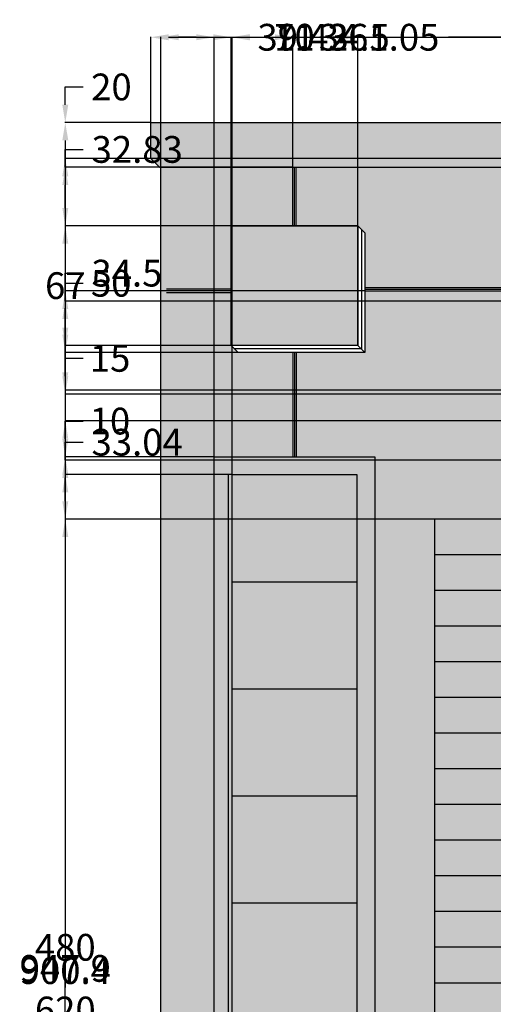
# Model space of a CAD drawing. Units: millimetres. Extents: x 131 to 845, y -20 to 1043.
# Tile 9 of 11: x 137 to 403, y 492 to 1043. Entities that reach past the tile are written whole.
import ezdxf

# ---------------------------------------------------------------- set-up
doc = ezdxf.new("R2010")
doc.units = ezdxf.units.MM
doc.header["$MEASUREMENT"] = 0
for name, color, linetype, lineweight in [('A-ANNO-DIMS', 2, 'Continuous', 18), ('A-ELEV', 7, 'Continuous', 25), ('A-ELEV-PATT', 7, 'Continuous', 13), ('A-GLAZ', 4, 'Continuous', 25), ('A-WALL-PATT', 131, 'Continuous', 13)]:
    doc.layers.add(name, color=color, linetype=linetype, lineweight=lineweight)
doc.styles.get("Standard").update_dxf_attribs({"font": 'arial.ttf'})
doc.dimstyles.get("Standard").update_dxf_attribs({"dimtxt": 15, "dimasz": 10, "dimexe": 0.18, "dimexo": 0.0625, "dimgap": 5, "dimtad": 0, "dimtih": 1, "dimtoh": 1, "dimdec": 0, "dimzin": 0, "dimdsep": 46, "dimtxsty": 'Standard', "dimcen": 5, "dimadec": 0, "dimazin": 0, "dimtfac": 1, "dimtdec": 0, "dimtofl": 0, "dimtmove": 0, "dimatfit": 3, "dimfxl": 1, "dimtolj": 1, "dimtzin": 0, "dimarcsym": 0})

# ---------------------------------------------------------------- blocks, each defined once
blk = doc.blocks.new('*U3')
blk.add_line((0, -70), (0, 0))
blk = doc.blocks.new('*U4')
at = {"layer": 'A-GLAZ', "color": 0, "linetype": 'ByBlock', "lineweight": -2, "transparency": 16777216, "rotation": 270}
for p in [(326.16, 788.43), (326.16, 728.43), (326.16, 668.43), (326.16, 608.43), (326.16, 548.43)]:
    blk.add_blockref('*U3', p, dxfattribs=at)
blk = doc.blocks.new('*U5')
blk.add_line((0, 90), (0, 0))
blk = doc.blocks.new('*U6')
at = {"layer": 'A-ELEV', "color": 0, "linetype": 'ByBlock', "lineweight": -2, "transparency": 16777216, "rotation": 270}
for p in [(369.56, 763.56), (369.56, 743.56), (369.56, 723.56), (369.56, 703.56), (369.56, 683.56), (369.56, 663.56), (369.56, 643.56), (369.56, 623.56), (369.56, 603.56), (369.56, 583.56), (369.56, 563.56), (369.56, 543.56), (369.56, 523.56), (369.56, 503.56), (369.56, 483.56), (369.56, 463.56), (369.56, 443.56), (369.56, 423.56), (369.56, 403.56), (369.56, 383.56), (369.56, 363.56), (369.56, 343.56), (369.56, 323.56), (369.56, 303.56), (369.56, 283.56)]:
    blk.add_blockref('*U5', p, dxfattribs=at)
blk = doc.blocks.new('*D11')
at = {"layer": 'A-ANNO-DIMS', "color": 0, "lineweight": -2, "transparency": 16777216}
for p, q in [((554.73, 464.78), (544.73, 464.78)), ((554.75, 454.78), (554.73, 464.78)), ((550.09, 454.77), (554.93, 454.78)), ((554.78, 433.28), (554.76, 444.78)), ((550.13, 423.27), (554.97, 423.28))]:
    blk.add_line(p, q, dxfattribs=at)
at = {"layer": 'A-ANNO-DIMS', "color": 0, "transparency": 16777216}
for points in [[(556.43, 444.78), (553.1, 444.77), (554.75, 454.78)], [(556.45, 433.28), (553.11, 433.27), (554.79, 423.28)]]:
    blk.add_solid(points, dxfattribs=at)
at = {"layer": 'Defpoints', "color": 0, "transparency": 16777216}
for p in [(550.02, 454.77), (554.75, 454.78), (550.07, 423.27)]:
    blk.add_point(p, dxfattribs=at)
at = {"layer": 'A-ANNO-DIMS', "color": 0, "transparency": 16777216, "insert": (399.96, 464.78), "char_height": 15, "attachment_point": 5}
blk.add_mtext('\\A1;DOOR GLASS PANE 32 TYP.', dxfattribs=at)
blk = doc.blocks.new('*D13')
at = {"layer": 'A-ANNO-DIMS', "color": 0, "lineweight": -2, "transparency": 16777216}
for p, q in [((210.58, 985.73), (210.58, 1033.7)), ((220.58, 1033.52), (444.01, 1033.52)), ((710.53, 1033.52), (487.1, 1033.52)), ((720.53, 818.66), (720.53, 1033.7))]:
    blk.add_line(p, q, dxfattribs=at)
at = {"layer": 'A-ANNO-DIMS', "color": 0, "transparency": 16777216}
for points in [[(220.58, 1035.18), (220.58, 1031.85), (210.58, 1033.52)], [(710.53, 1035.18), (710.53, 1031.85), (720.53, 1033.52)]]:
    blk.add_solid(points, dxfattribs=at)
at = {"layer": 'Defpoints', "color": 0, "transparency": 16777216}
for p in [(720.53, 1033.52), (210.58, 985.67), (720.53, 818.6)]:
    blk.add_point(p, dxfattribs=at)
at = {"layer": 'A-ANNO-DIMS', "color": 0, "transparency": 16777216, "insert": (465.56, 1033.52), "char_height": 15, "attachment_point": 5}
blk.add_mtext('\\A1;510', dxfattribs=at)
blk = doc.blocks.new('*D14')
at = {"layer": 'A-ANNO-DIMS', "color": 0, "lineweight": -2, "transparency": 16777216}
for p, q in [((210.52, 985.67), (162.55, 985.67)), ((162.73, 975.67), (162.73, 524.4)), ((162.73, 47.81), (162.73, 499.08)), ((459.5, 37.81), (162.55, 37.81))]:
    blk.add_line(p, q, dxfattribs=at)
at = {"layer": 'A-ANNO-DIMS', "color": 0, "transparency": 16777216}
for points in [[(161.06, 975.67), (164.4, 975.67), (162.73, 985.67)], [(161.06, 47.81), (164.4, 47.81), (162.73, 37.81)]]:
    blk.add_solid(points, dxfattribs=at)
at = {"layer": 'Defpoints', "color": 0, "transparency": 16777216}
for p in [(162.73, 985.67), (210.58, 985.67), (459.56, 37.81)]:
    blk.add_point(p, dxfattribs=at)
at = {"layer": 'A-ANNO-DIMS', "color": 0, "transparency": 16777216, "insert": (162.73, 511.74), "char_height": 15, "attachment_point": 5}
blk.add_mtext('\\A1;947.9', dxfattribs=at)
blk = doc.blocks.new('*D15')
at = {"layer": 'A-ANNO-DIMS', "color": 0, "lineweight": -2, "transparency": 16777216}
for p, q in [((210.58, 985.73), (210.58, 1033.7)), ((220.58, 1033.52), (304.79, 1033.52)), ((461.63, 1033.52), (377.43, 1033.52)), ((471.63, 965.73), (471.63, 1033.7))]:
    blk.add_line(p, q, dxfattribs=at)
at = {"layer": 'A-ANNO-DIMS', "color": 0, "transparency": 16777216}
for points in [[(220.58, 1035.18), (220.58, 1031.85), (210.58, 1033.52)], [(461.63, 1035.18), (461.63, 1031.85), (471.63, 1033.52)]]:
    blk.add_solid(points, dxfattribs=at)
at = {"layer": 'Defpoints', "color": 0, "transparency": 16777216}
for p in [(471.63, 1033.52), (210.58, 985.67), (471.63, 965.67)]:
    blk.add_point(p, dxfattribs=at)
at = {"layer": 'A-ANNO-DIMS', "color": 0, "transparency": 16777216, "insert": (341.11, 1033.52), "char_height": 15, "attachment_point": 5}
blk.add_mtext('\\A1;261.05', dxfattribs=at)
blk = doc.blocks.new('*D16')
at = {"layer": 'A-ANNO-DIMS', "color": 0, "lineweight": -2, "transparency": 16777216}
for p, q in [((162.73, 995.67), (162.73, 1005.67)), ((162.73, 1005.67), (172.73, 1005.67)), ((210.52, 985.67), (162.55, 985.67)), ((210.52, 965.67), (162.55, 965.67)), ((162.73, 955.67), (162.73, 945.67))]:
    blk.add_line(p, q, dxfattribs=at)
at = {"layer": 'A-ANNO-DIMS', "color": 0, "transparency": 16777216}
for points in [[(161.06, 995.67), (164.4, 995.67), (162.73, 985.67)], [(161.06, 955.67), (164.4, 955.67), (162.73, 965.67)]]:
    blk.add_solid(points, dxfattribs=at)
at = {"layer": 'Defpoints', "color": 0, "transparency": 16777216}
for p in [(162.73, 985.67), (210.58, 985.67), (210.58, 965.67)]:
    blk.add_point(p, dxfattribs=at)
at = {"layer": 'A-ANNO-DIMS', "color": 0, "transparency": 16777216, "insert": (188.58, 1005.67), "char_height": 15, "attachment_point": 5}
blk.add_mtext('\\A1;20', dxfattribs=at)
blk = doc.blocks.new('*D17')
at = {"layer": 'A-ANNO-DIMS', "color": 0, "lineweight": -2, "transparency": 16777216}
for p, q in [((216.17, 960.67), (162.55, 960.67)), ((162.73, 950.67), (162.73, 523.15)), ((162.73, 70.31), (162.73, 497.83)), ((216.17, 60.31), (162.55, 60.31))]:
    blk.add_line(p, q, dxfattribs=at)
at = {"layer": 'A-ANNO-DIMS', "color": 0, "transparency": 16777216}
for points in [[(161.06, 950.67), (164.4, 950.67), (162.73, 960.67)], [(161.06, 70.31), (164.4, 70.31), (162.73, 60.31)]]:
    blk.add_solid(points, dxfattribs=at)
at = {"layer": 'Defpoints', "color": 0, "transparency": 16777216}
for p in [(162.73, 960.67), (216.23, 960.67), (216.23, 60.31)]:
    blk.add_point(p, dxfattribs=at)
at = {"layer": 'A-ANNO-DIMS', "color": 0, "transparency": 16777216, "insert": (162.73, 510.49), "char_height": 15, "attachment_point": 5}
blk.add_mtext('\\A1;900.4', dxfattribs=at)
blk = doc.blocks.new('*D19')
at = {"layer": 'A-ANNO-DIMS', "color": 0, "lineweight": -2, "transparency": 16777216}
for p, q in [((216.23, 960.73), (216.23, 1033.7)), ((226.23, 1033.52), (245.66, 1033.52)), ((255.66, 927.9), (255.66, 1033.7)), ((255.66, 1033.52), (265.66, 1033.52))]:
    blk.add_line(p, q, dxfattribs=at)
at = {"layer": 'A-ANNO-DIMS', "color": 0, "transparency": 16777216}
for points in [[(226.23, 1035.18), (226.23, 1031.85), (216.23, 1033.52)], [(245.66, 1035.18), (245.66, 1031.85), (255.66, 1033.52)]]:
    blk.add_solid(points, dxfattribs=at)
at = {"layer": 'Defpoints', "color": 0, "transparency": 16777216}
for p in [(255.66, 1033.52), (216.23, 960.67), (255.66, 927.83)]:
    blk.add_point(p, dxfattribs=at)
at = {"layer": 'A-ANNO-DIMS', "color": 0, "transparency": 16777216, "insert": (295.96, 1033.52), "char_height": 15, "attachment_point": 5}
blk.add_mtext('\\A1;39.43', dxfattribs=at)
blk = doc.blocks.new('*D20')
at = {"layer": 'A-ANNO-DIMS', "color": 0, "lineweight": -2, "transparency": 16777216}
for p, q in [((255.66, 860.9), (255.66, 1033.7)), ((265.66, 1033.52), (276.93, 1033.52)), ((316.66, 1033.52), (305.39, 1033.52)), ((326.66, 860.9), (326.66, 1033.7))]:
    blk.add_line(p, q, dxfattribs=at)
at = {"layer": 'A-ANNO-DIMS', "color": 0, "transparency": 16777216}
for points in [[(265.66, 1035.18), (265.66, 1031.85), (255.66, 1033.52)], [(316.66, 1035.18), (316.66, 1031.85), (326.66, 1033.52)]]:
    blk.add_solid(points, dxfattribs=at)
at = {"layer": 'Defpoints', "color": 0, "transparency": 16777216}
for p in [(326.66, 1033.52), (255.66, 860.83), (326.66, 860.83)]:
    blk.add_point(p, dxfattribs=at)
at = {"layer": 'A-ANNO-DIMS', "color": 0, "transparency": 16777216, "insert": (291.16, 1033.52), "char_height": 15, "attachment_point": 5}
blk.add_mtext('\\A1;71', dxfattribs=at)
blk = doc.blocks.new('*D21')
at = {"layer": 'A-ANNO-DIMS', "color": 0, "lineweight": -2, "transparency": 16777216}
for p, q in [((326.6, 927.83), (162.55, 927.83)), ((162.73, 917.83), (162.73, 906.99)), ((162.73, 870.83), (162.73, 881.68)), ((326.6, 860.83), (162.55, 860.83))]:
    blk.add_line(p, q, dxfattribs=at)
at = {"layer": 'A-ANNO-DIMS', "color": 0, "transparency": 16777216}
for points in [[(161.06, 917.83), (164.4, 917.83), (162.73, 927.83)], [(161.06, 870.83), (164.4, 870.83), (162.73, 860.83)]]:
    blk.add_solid(points, dxfattribs=at)
at = {"layer": 'Defpoints', "color": 0, "transparency": 16777216}
for p in [(162.73, 927.83), (326.66, 927.83), (326.66, 860.83)]:
    blk.add_point(p, dxfattribs=at)
at = {"layer": 'A-ANNO-DIMS', "color": 0, "transparency": 16777216, "insert": (162.73, 894.33), "char_height": 15, "attachment_point": 5}
blk.add_mtext('\\A1;67', dxfattribs=at)
blk = doc.blocks.new('*D22')
at = {"layer": 'A-ANNO-DIMS', "color": 0, "lineweight": -2, "transparency": 16777216}
for p, q in [((162.73, 960.67), (162.73, 970.67)), ((162.73, 970.67), (172.73, 970.67)), ((290.1, 960.67), (162.55, 960.67)), ((162.73, 937.83), (162.73, 950.67)), ((326.6, 927.83), (162.55, 927.83))]:
    blk.add_line(p, q, dxfattribs=at)
at = {"layer": 'A-ANNO-DIMS', "color": 0, "transparency": 16777216}
for points in [[(161.06, 950.67), (164.4, 950.67), (162.73, 960.67)], [(161.06, 937.83), (164.4, 937.83), (162.73, 927.83)]]:
    blk.add_solid(points, dxfattribs=at)
at = {"layer": 'Defpoints', "color": 0, "transparency": 16777216}
for p in [(162.73, 960.67), (290.16, 960.67), (326.66, 927.83)]:
    blk.add_point(p, dxfattribs=at)
at = {"layer": 'A-ANNO-DIMS', "color": 0, "transparency": 16777216, "insert": (203.04, 970.67), "char_height": 15, "attachment_point": 5}
blk.add_mtext('\\A1;32.83', dxfattribs=at)
blk = doc.blocks.new('*D23')
at = {"layer": 'A-ANNO-DIMS', "color": 0, "lineweight": -2, "transparency": 16777216}
for p, q in [((255.66, 927.9), (255.66, 1033.7)), ((265.66, 1033.52), (280.16, 1033.52)), ((290.16, 927.9), (290.16, 1033.7)), ((290.16, 1033.52), (300.16, 1033.52))]:
    blk.add_line(p, q, dxfattribs=at)
at = {"layer": 'A-ANNO-DIMS', "color": 0, "transparency": 16777216}
for points in [[(265.66, 1035.18), (265.66, 1031.85), (255.66, 1033.52)], [(280.16, 1035.18), (280.16, 1031.85), (290.16, 1033.52)]]:
    blk.add_solid(points, dxfattribs=at)
at = {"layer": 'Defpoints', "color": 0, "transparency": 16777216}
for p in [(290.16, 1033.52), (255.66, 927.83), (290.16, 927.83)]:
    blk.add_point(p, dxfattribs=at)
at = {"layer": 'A-ANNO-DIMS', "color": 0, "transparency": 16777216, "insert": (324.69, 1033.52), "char_height": 15, "attachment_point": 5}
blk.add_mtext('\\A1;34.5', dxfattribs=at)
blk = doc.blocks.new('*D24')
at = {"layer": 'A-ANNO-DIMS', "color": 0, "lineweight": -2, "transparency": 16777216}
for p, q in [((162.73, 891.33), (162.73, 901.33)), ((162.73, 901.33), (172.73, 901.33)), ((330.6, 891.33), (162.55, 891.33)), ((162.73, 866.83), (162.73, 881.33)), ((330.6, 856.83), (162.55, 856.83))]:
    blk.add_line(p, q, dxfattribs=at)
at = {"layer": 'A-ANNO-DIMS', "color": 0, "transparency": 16777216}
for points in [[(161.06, 881.33), (164.4, 881.33), (162.73, 891.33)], [(161.06, 866.83), (164.4, 866.83), (162.73, 856.83)]]:
    blk.add_solid(points, dxfattribs=at)
at = {"layer": 'Defpoints', "color": 0, "transparency": 16777216}
for p in [(162.73, 891.33), (330.66, 891.33), (330.66, 856.83)]:
    blk.add_point(p, dxfattribs=at)
at = {"layer": 'A-ANNO-DIMS', "color": 0, "transparency": 16777216, "insert": (197.26, 901.33), "char_height": 15, "attachment_point": 5}
blk.add_mtext('\\A1;34.5', dxfattribs=at)
blk = doc.blocks.new('*D28')
at = {"layer": 'A-ANNO-DIMS', "color": 0, "lineweight": -2, "transparency": 16777216}
for p, q in [((246.1, 798.43), (162.55, 798.43)), ((162.73, 788.43), (162.73, 501.09)), ((162.73, 188.43), (162.73, 475.77)), ((246.1, 178.43), (162.55, 178.43))]:
    blk.add_line(p, q, dxfattribs=at)
at = {"layer": 'A-ANNO-DIMS', "color": 0, "transparency": 16777216}
for points in [[(161.06, 788.43), (164.4, 788.43), (162.73, 798.43)], [(161.06, 188.43), (164.4, 188.43), (162.73, 178.43)]]:
    blk.add_solid(points, dxfattribs=at)
at = {"layer": 'Defpoints', "color": 0, "transparency": 16777216}
for p in [(162.73, 798.43), (246.16, 798.43), (246.16, 178.43)]:
    blk.add_point(p, dxfattribs=at)
at = {"layer": 'A-ANNO-DIMS', "color": 0, "transparency": 16777216, "insert": (162.73, 488.43), "char_height": 15, "attachment_point": 5}
blk.add_mtext('\\A1;620', dxfattribs=at)
blk = doc.blocks.new('*D30')
at = {"layer": 'A-ANNO-DIMS', "color": 0, "lineweight": -2, "transparency": 16777216}
for p, q in [((236.16, 1033.52), (226.16, 1033.52)), ((246.16, 798.5), (246.16, 1033.7)), ((256.16, 788.5), (256.16, 1033.7)), ((266.16, 1033.52), (276.16, 1033.52))]:
    blk.add_line(p, q, dxfattribs=at)
at = {"layer": 'A-ANNO-DIMS', "color": 0, "transparency": 16777216}
for points in [[(236.16, 1035.18), (236.16, 1031.85), (246.16, 1033.52)], [(266.16, 1035.18), (266.16, 1031.85), (256.16, 1033.52)]]:
    blk.add_solid(points, dxfattribs=at)
at = {"layer": 'Defpoints', "color": 0, "transparency": 16777216}
for p in [(256.16, 1033.52), (246.16, 798.43), (256.16, 788.43)]:
    blk.add_point(p, dxfattribs=at)
at = {"layer": 'A-ANNO-DIMS', "color": 0, "transparency": 16777216, "insert": (291.17, 1033.52), "char_height": 15, "attachment_point": 5}
blk.add_mtext('\\A1;10', dxfattribs=at)
blk = doc.blocks.new('*D31')
at = {"layer": 'A-ANNO-DIMS', "color": 0, "lineweight": -2, "transparency": 16777216}
for p, q in [((162.73, 808.43), (162.73, 818.43)), ((162.73, 818.43), (172.73, 818.43)), ((246.1, 798.43), (162.55, 798.43)), ((256.1, 788.43), (162.55, 788.43)), ((162.73, 778.43), (162.73, 768.43))]:
    blk.add_line(p, q, dxfattribs=at)
at = {"layer": 'A-ANNO-DIMS', "color": 0, "transparency": 16777216}
for points in [[(161.06, 808.43), (164.4, 808.43), (162.73, 798.43)], [(161.06, 778.43), (164.4, 778.43), (162.73, 788.43)]]:
    blk.add_solid(points, dxfattribs=at)
at = {"layer": 'Defpoints', "color": 0, "transparency": 16777216}
for p in [(162.73, 798.43), (246.16, 798.43), (256.16, 788.43)]:
    blk.add_point(p, dxfattribs=at)
at = {"layer": 'A-ANNO-DIMS', "color": 0, "transparency": 16777216, "insert": (187.74, 818.43), "char_height": 15, "attachment_point": 5}
blk.add_mtext('\\A1;10', dxfattribs=at)
blk = doc.blocks.new('*D35')
at = {"layer": 'A-ANNO-DIMS', "color": 0, "lineweight": -2, "transparency": 16777216}
for p, q in [((369.5, 763.56), (162.55, 763.56)), ((162.73, 753.56), (162.73, 536.21)), ((162.73, 293.56), (162.73, 510.9)), ((369.5, 283.56), (162.55, 283.56))]:
    blk.add_line(p, q, dxfattribs=at)
at = {"layer": 'A-ANNO-DIMS', "color": 0, "transparency": 16777216}
for points in [[(161.06, 753.56), (164.4, 753.56), (162.73, 763.56)], [(161.06, 293.56), (164.4, 293.56), (162.73, 283.56)]]:
    blk.add_solid(points, dxfattribs=at)
at = {"layer": 'Defpoints', "color": 0, "transparency": 16777216}
for p in [(162.73, 763.56), (369.56, 763.56), (369.56, 283.56)]:
    blk.add_point(p, dxfattribs=at)
at = {"layer": 'A-ANNO-DIMS', "color": 0, "transparency": 16777216, "insert": (162.73, 523.56), "char_height": 15, "attachment_point": 5}
blk.add_mtext('\\A1;480', dxfattribs=at)
blk = doc.blocks.new('*D45')
at = {"layer": 'A-ANNO-DIMS', "color": 0, "lineweight": -2, "transparency": 16777216}
for p, q in [((162.73, 796.6), (162.73, 806.6)), ((162.73, 806.6), (172.73, 806.6)), ((439.5, 796.6), (162.55, 796.6)), ((162.73, 773.56), (162.73, 786.6)), ((459.5, 763.56), (162.55, 763.56))]:
    blk.add_line(p, q, dxfattribs=at)
at = {"layer": 'A-ANNO-DIMS', "color": 0, "transparency": 16777216}
for points in [[(161.06, 786.6), (164.4, 786.6), (162.73, 796.6)], [(161.06, 773.56), (164.4, 773.56), (162.73, 763.56)]]:
    blk.add_solid(points, dxfattribs=at)
at = {"layer": 'Defpoints', "color": 0, "transparency": 16777216}
for p in [(162.73, 796.6), (439.56, 796.6), (459.56, 763.56)]:
    blk.add_point(p, dxfattribs=at)
at = {"layer": 'A-ANNO-DIMS', "color": 0, "transparency": 16777216, "insert": (203, 806.6), "char_height": 15, "attachment_point": 5}
blk.add_mtext('\\A1;33.04', dxfattribs=at)
blk = doc.blocks.new('*D93')
at = {"layer": 'A-ANNO-DIMS', "color": 0, "lineweight": -2, "transparency": 16777216}
for p, q in [((162.73, 843.6), (162.73, 853.6)), ((162.73, 853.6), (172.73, 853.6)), ((449.5, 833.6), (162.55, 833.6)), ((449.5, 818.6), (162.55, 818.6)), ((162.73, 808.6), (162.73, 798.6))]:
    blk.add_line(p, q, dxfattribs=at)
at = {"layer": 'A-ANNO-DIMS', "color": 0, "transparency": 16777216}
for points in [[(161.06, 843.6), (164.4, 843.6), (162.73, 833.6)], [(161.06, 808.6), (164.4, 808.6), (162.73, 818.6)]]:
    blk.add_solid(points, dxfattribs=at)
at = {"layer": 'Defpoints', "color": 0, "transparency": 16777216}
for p in [(162.73, 833.6), (449.56, 833.6), (449.56, 818.6)]:
    blk.add_point(p, dxfattribs=at)
at = {"layer": 'A-ANNO-DIMS', "color": 0, "transparency": 16777216, "insert": (187.83, 853.6), "char_height": 15, "attachment_point": 5}
blk.add_mtext('\\A1;15', dxfattribs=at)
blk = doc.blocks.new('*D94')
at = {"layer": 'A-ANNO-DIMS', "color": 0, "lineweight": -2, "transparency": 16777216}
for p, q in [((162.73, 885.67), (162.73, 895.67)), ((162.73, 895.67), (172.73, 895.67)), ((451.57, 885.67), (162.55, 885.67)), ((162.73, 845.67), (162.73, 875.67)), ((451.57, 835.67), (162.55, 835.67))]:
    blk.add_line(p, q, dxfattribs=at)
at = {"layer": 'A-ANNO-DIMS', "color": 0, "transparency": 16777216}
for points in [[(161.06, 875.67), (164.4, 875.67), (162.73, 885.67)], [(161.06, 845.67), (164.4, 845.67), (162.73, 835.67)]]:
    blk.add_solid(points, dxfattribs=at)
at = {"layer": 'Defpoints', "color": 0, "transparency": 16777216}
for p in [(162.73, 885.67), (451.63, 885.67), (451.63, 835.67)]:
    blk.add_point(p, dxfattribs=at)
at = {"layer": 'A-ANNO-DIMS', "color": 0, "transparency": 16777216, "insert": (188.45, 895.67), "char_height": 15, "attachment_point": 5}
blk.add_mtext('\\A1;50', dxfattribs=at)

msp = doc.modelspace()

# ---------------------------------------------------------------- hatches: boundary and pattern name
at = {"layer": 'A-ELEV-PATT'}
h = msp.add_hatch(color=256, dxfattribs=at)
h.set_gradient(color1=(255, 255, 255), color2=(99, 100, 102), name='INVSPHERICAL')
h.paths.add_polyline_path([(471.6297, 965.6663), (471.6297, 980.6663), (466.6297, 985.6663), (210.5817, 985.6663), (210.5817, 965.6663)])
h = msp.add_hatch(color=256, dxfattribs=at)
h.set_gradient(color1=(255, 255, 255), color2=(99, 100, 102))
h.paths.add_polyline_path([(210.5817, 965.6663), (215.5817, 960.6663), (466.6297, 960.6663), (466.6297, 885.6663), (471.6297, 885.6663), (471.6297, 960.6663), (471.6297, 965.6663)])
h = msp.add_hatch(color=256, dxfattribs=at)
h.set_gradient(color1=(199, 200, 202), color2=(99, 100, 102), name='SPHERICAL')
h.paths.add_polyline_path([(255.6595, 927.8345), (255.6595, 860.8345), (326.6595, 860.8345), (326.6595, 927.8345)])
h.paths.add_polyline_path([(336.1595, 798.4332), (246.1595, 798.4332), (246.1595, 178.4332), (336.1595, 178.4332), (336.1595, 186.4332), (254.1595, 186.4332), (254.1595, 788.4332), (256.1595, 788.4332), (326.1595, 788.4332), (326.1595, 188.4332), (256.1595, 188.4332), (256.1595, 788.4332), (254.1595, 788.4332), (254.1595, 186.4332), (336.1595, 186.4332), (336.1595, 188.4332)])
h = msp.add_hatch(color=256, dxfattribs=at)
h.set_gradient(color1=(199, 200, 202), color2=(255, 255, 0), name='INVCYLINDER')
h.paths.add_polyline_path([(326.1595, 728.4332), (326.1595, 788.4332), (256.1595, 788.4332), (256.1595, 728.4332)])
h.paths.add_polyline_path([(326.1595, 668.4332), (326.1595, 728.4332), (256.1595, 728.4332), (256.1595, 668.4332)])
h.paths.add_polyline_path([(326.1595, 608.4332), (326.1595, 668.4332), (256.1595, 668.4332), (256.1595, 608.4332)])
h.paths.add_polyline_path([(326.1595, 548.4332), (326.1595, 608.4332), (256.1595, 608.4332), (256.1595, 548.4332)])
h.paths.add_polyline_path([(326.1595, 488.4332), (326.1595, 548.4332), (256.1595, 548.4332), (256.1595, 488.4332)])
h.paths.add_polyline_path([(326.1595, 428.4332), (326.1595, 488.4332), (256.1595, 488.4332), (256.1595, 428.4332)])
h.paths.add_polyline_path([(326.1595, 368.4332), (326.1595, 428.4332), (256.1595, 428.4332), (256.1595, 368.4332)])
h.paths.add_polyline_path([(256.1595, 368.4332), (256.1595, 308.4332), (326.1595, 308.4332), (326.1595, 368.4332)])
h.paths.add_polyline_path([(256.1595, 308.4332), (256.1595, 248.4332), (326.1595, 248.4332), (326.1595, 308.4332)])
h.paths.add_polyline_path([(256.1595, 248.4332), (256.1595, 188.4332), (326.1595, 188.4332), (326.1595, 248.4332)])
at = {"layer": 'A-ELEV-PATT', "transparency": 33554681}
h = msp.add_hatch(color=256, dxfattribs=at)
h.set_gradient(color1=(147, 149, 152), color2=(192, 192, 192), name='CYLINDER')
h.paths.add_polyline_path([(369.5586, 763.5561), (369.5586, 743.5561), (459.5586, 743.5561), (459.5586, 763.5561)])
h.paths.add_polyline_path([(459.5586, 703.5561), (459.5586, 723.5561), (369.5586, 723.5561), (369.5586, 703.5561)])
h.paths.add_polyline_path([(459.5586, 663.5561), (459.5586, 683.5561), (369.5586, 683.5561), (369.5586, 663.5561)])
h.paths.add_polyline_path([(459.5586, 623.5561), (459.5586, 643.5561), (369.5586, 643.5561), (369.5586, 623.5561)])
h.paths.add_polyline_path([(459.5586, 583.5561), (459.5586, 603.5561), (369.5586, 603.5561), (369.5586, 583.5561)])
h.paths.add_polyline_path([(459.5586, 543.5561), (459.5586, 563.5561), (369.5586, 563.5561), (369.5586, 543.5561)])
h.paths.add_polyline_path([(369.5586, 523.5561), (369.5586, 503.5561), (409.6606, 503.5561), (409.6606, 503.5953), (412.6606, 503.5953), (412.6606, 513.5953), (414.417, 523.5561)])
h.paths.add_polyline_path([(369.5586, 483.5561), (369.5586, 463.5561), (459.5586, 463.5561), (459.5586, 483.5561)])
h.paths.add_polyline_path([(459.5586, 423.5561), (459.5586, 443.5561), (369.5586, 443.5561), (369.5586, 423.5561)])
h.paths.add_polyline_path([(369.5586, 403.5561), (369.5586, 383.5561), (459.5586, 383.5561), (459.5586, 403.5561)])
h.paths.add_polyline_path([(459.5586, 343.5561), (459.5586, 363.5561), (369.5586, 363.5561), (369.5586, 343.5561)])
h.paths.add_polyline_path([(369.5586, 323.5561), (369.5586, 303.5561), (459.5586, 303.5561), (459.5586, 323.5561)])
h = msp.add_hatch(color=256, dxfattribs=at)
h.set_gradient(color1=(147, 149, 152), color2=(192, 192, 192), name='CURVED')
h.paths.add_polyline_path([(369.5586, 743.5561), (369.5586, 723.5561), (459.5586, 723.5561), (459.5586, 743.5561)])
h.paths.add_polyline_path([(369.5586, 703.5561), (369.5586, 683.5561), (459.5586, 683.5561), (459.5586, 703.5561)])
h.paths.add_polyline_path([(459.5586, 643.5561), (459.5586, 663.5561), (369.5586, 663.5561), (369.5586, 643.5561)])
h.paths.add_polyline_path([(459.5586, 603.5561), (459.5586, 623.5561), (369.5586, 623.5561), (369.5586, 603.5561)])
h.paths.add_polyline_path([(369.5586, 583.5561), (369.5586, 563.5561), (459.5586, 563.5561), (459.5586, 583.5561)])
h.paths.add_polyline_path([(369.5586, 543.5561), (369.5586, 523.5561), (459.5586, 523.5561), (459.5586, 543.5561)])
h.paths.add_polyline_path([(459.5586, 483.5561), (459.5586, 488.5953), (412.6606, 488.5953), (412.6606, 498.5953), (409.6606, 498.5953), (409.6606, 503.5561), (369.5586, 503.5561), (369.5586, 483.5561)])
h.paths.add_polyline_path([(369.5586, 463.5561), (369.5586, 443.5561), (459.5586, 443.5561), (459.5586, 463.5561)])
h.paths.add_polyline_path([(369.5586, 423.5561), (369.5586, 403.5561), (459.5586, 403.5561), (459.5586, 423.5561)])
h.paths.add_polyline_path([(369.5586, 383.5561), (369.5586, 363.5561), (459.5586, 363.5561), (459.5586, 383.5561)])
h.paths.add_polyline_path([(369.5586, 343.5561), (369.5586, 323.5561), (459.5586, 323.5561), (459.5586, 343.5561)])
h.paths.add_polyline_path([(369.5586, 303.5561), (369.5586, 283.5561), (459.5586, 283.5561), (459.5586, 303.5561)])
at = {"layer": 'A-WALL-PATT'}
h = msp.add_hatch(color=256, dxfattribs=at)
h.dxf.hatch_style = 1
h.paths.add_polyline_path([(449.5586, 833.5953), (451.6297, 835.6663), (451.6297, 885.6663), (466.6297, 885.6663), (466.6297, 891.3345), (330.6595, 891.3345), (330.6595, 856.8345), (292.1595, 856.8345), (292.1595, 798.4332), (336.1595, 798.4332), (336.1595, 178.4332), (246.1595, 178.4332), (246.1595, 798.4332), (290.1595, 798.4332), (290.1595, 856.8345), (259.6595, 856.8345), (255.6595, 860.8345), (255.6595, 927.8345), (290.1595, 927.8345), (290.1595, 960.6663), (216.2327, 960.6663), (216.2327, 60.3131), (459.5586, 60.3131), (459.5586, 97.8131), (459.5586, 252.07), (459.5586, 283.5561), (369.5586, 283.5561), (369.5586, 763.5561), (439.5586, 763.5561), (439.5586, 778.6714), (439.5586, 793.5953), (439.5586, 796.5953), (441.5586, 798.5953), (444.5586, 798.5953), (444.5586, 813.5953), (444.5586, 816.5953), (446.5586, 818.5953), (449.5586, 818.5953)])
h.paths.add_polyline_path([(466.6297, 960.6663), (292.1595, 960.6663), (292.1595, 927.8345), (326.6595, 927.8345), (330.6595, 923.8345), (330.6595, 893.3345), (466.6297, 893.3345)], flags=17)
h.paths.add_polyline_path([(720.5349, 813.5953), (720.5349, 818.5953), (710.5349, 818.5953), (449.5586, 818.5953), (446.5586, 818.5953), (444.5586, 816.5953), (444.5586, 813.5953), (444.5586, 798.5953), (705.5349, 798.5953), (705.5349, 513.5953), (705.5349, 498.5953), (680.5349, 498.5953), (680.5349, 488.5953), (705.5349, 488.5953), (720.5349, 488.5953), (720.5349, 513.5953)])
h.paths.add_polyline_path([(680.5349, 498.5953), (412.6606, 498.5953), (412.6606, 488.5953), (680.5349, 488.5953)])

# ---------------------------------------------------------------- linework, layer by layer
at = {"layer": 'A-ELEV'}
for p, q in [((210.5817, 965.6663), (210.5817, 985.6663)), ((210.5817, 985.6663), (466.6297, 985.6663)), ((471.6297, 965.6663), (210.5817, 965.6663)), ((210.5817, 965.6663), (215.5817, 960.6663)), ((215.5817, 960.6663), (466.6297, 960.6663)), ((216.2327, 60.3131), (216.2327, 960.6663)), ((290.1595, 927.8345), (290.1595, 960.6663)), ((291.1595, 927.8345), (291.1595, 960.6663)), ((291.1595, 927.8345), (291.1595, 960.6663)), ((292.1595, 927.8345), (292.1595, 960.6663)), ((255.6595, 860.8345), (255.6595, 927.8345)), ((255.6595, 927.8345), (326.6595, 927.8345)), ((326.6595, 927.8345), (326.6595, 860.8345)), ((326.6595, 927.8345), (330.6595, 923.8345)), ((328.6595, 925.8345), (328.6595, 858.8345)), ((330.6595, 923.8345), (330.6595, 856.8345)), ((255.6595, 892.3345), (219.4114, 892.3345)), ((255.6595, 891.3345), (219.4114, 891.3345)), ((255.6595, 890.3345), (219.4114, 890.3345)), ((330.6595, 893.3345), (466.6297, 893.3345)), ((330.6595, 892.3345), (466.6297, 892.3345)), ((330.6595, 891.3345), (466.6297, 891.3345)), ((326.6595, 860.8345), (255.6595, 860.8345)), ((255.6595, 860.8345), (259.6595, 856.8345)), ((326.6595, 860.8345), (330.6595, 856.8345)), ((328.6595, 858.8345), (257.6595, 858.8345)), ((330.6595, 856.8345), (259.6595, 856.8345)), ((290.1595, 856.8345), (290.1595, 798.4332)), ((291.1595, 856.8345), (291.1595, 798.4332)), ((292.1595, 856.8345), (292.1595, 798.4332)), ((292.1595, 856.8345), (292.1595, 798.4332)), ((246.1595, 798.4332), (336.1595, 798.4332)), ((246.1595, 178.4332), (246.1595, 798.4332)), ((336.1595, 798.4332), (336.1595, 178.4332)), ((254.1595, 186.4332), (254.1595, 788.4332)), ((256.1595, 788.4332), (254.1595, 788.4332)), ((256.1595, 188.4332), (256.1595, 788.4332)), ((326.1595, 788.4332), (326.1595, 188.4332)), ((369.5586, 763.5561), (369.5586, 283.5561))]:
    msp.add_line(p, q, dxfattribs=at)

# ---------------------------------------------------------------- block references
msp.add_blockref('*U6', (0, 0), dxfattribs=at)
at = {"layer": 'A-GLAZ'}
msp.add_blockref('*U4', (0, 0), dxfattribs=at)

# ---------------------------------------------------------------- dimensions: what is measured, and where the dimension line sits
at = {"layer": 'A-ANNO-DIMS'}
for base, p1, p2, override, picture, middle in [((720.5349, 1033.5163), (210.5817, 985.6663), (720.5349, 818.5953), {"dimdec": 0, "dimlfac": 1, "dimrnd": 0, "dimzin": 0, "dimdsep": 46, "dimlunit": 2}, '*D13', (465.5583, 1033.5163)), ((471.6297, 1033.5163), (210.5817, 985.6663), (471.6297, 965.6663), {"dimdec": 2, "dimlfac": 1, "dimrnd": 0, "dimzin": 0, "dimdsep": 46, "dimlunit": 2}, '*D15', (341.1057, 1033.5163)), ((255.6595, 1033.5163), (216.2327, 960.6663), (255.6595, 927.8345), {"dimdec": 2, "dimlfac": 1, "dimrnd": 0, "dimzin": 0, "dimdsep": 46, "dimlunit": 2}, '*D19', (295.9631, 1033.5163)), ((256.1595, 1033.5163), (246.1595, 798.4332), (256.1595, 788.4332), {"dimdec": 0, "dimlfac": 1, "dimrnd": 0, "dimzin": 0, "dimdsep": 46, "dimlunit": 2}, '*D30', (291.1715, 1033.5163)), ((326.6595, 1033.5163), (255.6595, 860.8345), (326.6595, 860.8345), {"dimdec": 0, "dimlfac": 1, "dimrnd": 0, "dimzin": 0, "dimdsep": 46, "dimlunit": 2}, '*D20', (291.1595, 1033.5163)), ((290.1595, 1033.5163), (255.6595, 927.8345), (290.1595, 927.8345), {"dimdec": 1, "dimlfac": 1, "dimrnd": 0, "dimzin": 0, "dimdsep": 46, "dimlunit": 2}, '*D23', (324.6923, 1033.5163))]:
    dim = msp.add_linear_dim(base=base, p1=p1, p2=p2, dimstyle='Standard', override=override, dxfattribs=at)
    dim.commit()
    dim.dimension.update_dxf_attribs({"geometry": picture, "text_midpoint": middle})
for base, p1, p2, override, picture, middle in [((162.7317, 985.6663), (210.5817, 965.6663), (210.5817, 985.6663), {"dimdec": 0, "dimlfac": 1, "dimrnd": 0, "dimzin": 0, "dimdsep": 46, "dimlunit": 2}, '*D16', (188.5775, 1005.6663)), ((162.7317, 985.6663), (459.5586, 37.8131), (210.5817, 985.6663), {"dimdec": 1, "dimlfac": 1, "dimrnd": 0, "dimzin": 0, "dimdsep": 46, "dimlunit": 2}, '*D14', (162.7317, 511.7397)), ((162.7317, 960.6663), (326.6595, 927.8345), (290.1595, 960.6663), {"dimdec": 2, "dimlfac": 1, "dimrnd": 0, "dimzin": 0, "dimdsep": 46, "dimlunit": 2}, '*D22', (203.0352, 970.6663)), ((162.7317, 960.6663), (216.2327, 60.3131), (216.2327, 960.6663), {"dimdec": 1, "dimlfac": 1, "dimrnd": 0, "dimzin": 0, "dimdsep": 46, "dimlunit": 2}, '*D17', (162.7317, 510.4897)), ((162.7317, 927.8345), (326.6595, 860.8345), (326.6595, 927.8345), {"dimdec": 0, "dimlfac": 1, "dimrnd": 0, "dimzin": 0, "dimdsep": 46, "dimlunit": 2}, '*D21', (162.7317, 894.3345)), ((162.7317, 891.3345), (330.6595, 856.8345), (330.6595, 891.3345), {"dimdec": 1, "dimlfac": 1, "dimrnd": 0, "dimzin": 0, "dimdsep": 46, "dimlunit": 2}, '*D24', (197.2644, 901.3345)), ((162.7317, 885.6663), (451.6297, 835.6663), (451.6297, 885.6663), {"dimdec": 0, "dimlfac": 1, "dimrnd": 0, "dimzin": 0, "dimdsep": 46, "dimlunit": 2}, '*D94', (188.4496, 895.6663)), ((162.7317, 833.5953), (449.5586, 818.5953), (449.5586, 833.5953), {"dimdec": 0, "dimlfac": 1, "dimrnd": 0, "dimzin": 0, "dimdsep": 46, "dimlunit": 2}, '*D93', (187.8254, 853.5953)), ((162.7317, 798.4332), (256.1595, 788.4332), (246.1595, 798.4332), {"dimdec": 0, "dimlfac": 1, "dimrnd": 0, "dimzin": 0, "dimdsep": 46, "dimlunit": 2}, '*D31', (187.7436, 818.4332)), ((162.7317, 796.5953), (459.5586, 763.5561), (439.5586, 796.5953), {"dimdec": 2, "dimlfac": 1, "dimrnd": 0, "dimzin": 0, "dimdsep": 46, "dimlunit": 2}, '*D45', (203.0045, 806.5953)), ((162.7317, 798.4332), (246.1595, 178.4332), (246.1595, 798.4332), {"dimdec": 0, "dimlfac": 1, "dimrnd": 0, "dimzin": 0, "dimdsep": 46, "dimlunit": 2}, '*D28', (162.7317, 488.4332)), ((162.7317, 763.5561), (369.5586, 283.5561), (369.5586, 763.5561), {"dimdec": 0, "dimlfac": 1, "dimrnd": 0, "dimzin": 0, "dimdsep": 46, "dimlunit": 2}, '*D35', (162.7317, 523.5561))]:
    dim = msp.add_linear_dim(base=base, p1=p1, p2=p2, angle=90, dimstyle='Standard', override=override, dxfattribs=at)
    dim.commit()
    dim.dimension.update_dxf_attribs({"geometry": picture, "text_midpoint": middle})
dim = msp.add_linear_dim(base=(554.7491, 454.7757), p1=(550.0694, 423.2689), p2=(550.0241, 454.7689), angle=90.082356, text='DOOR GLASS PANE <> TYP.', dimstyle='Standard', override={"dimdec": 0, "dimrnd": 0, "dimzin": 0, "dimlunit": 2}, dxfattribs=at)
dim.commit()
dim.dimension.update_dxf_attribs({"geometry": '*D11', "text_midpoint": (399.9615, 464.7756)})

doc.saveas('drawing.dxf')
